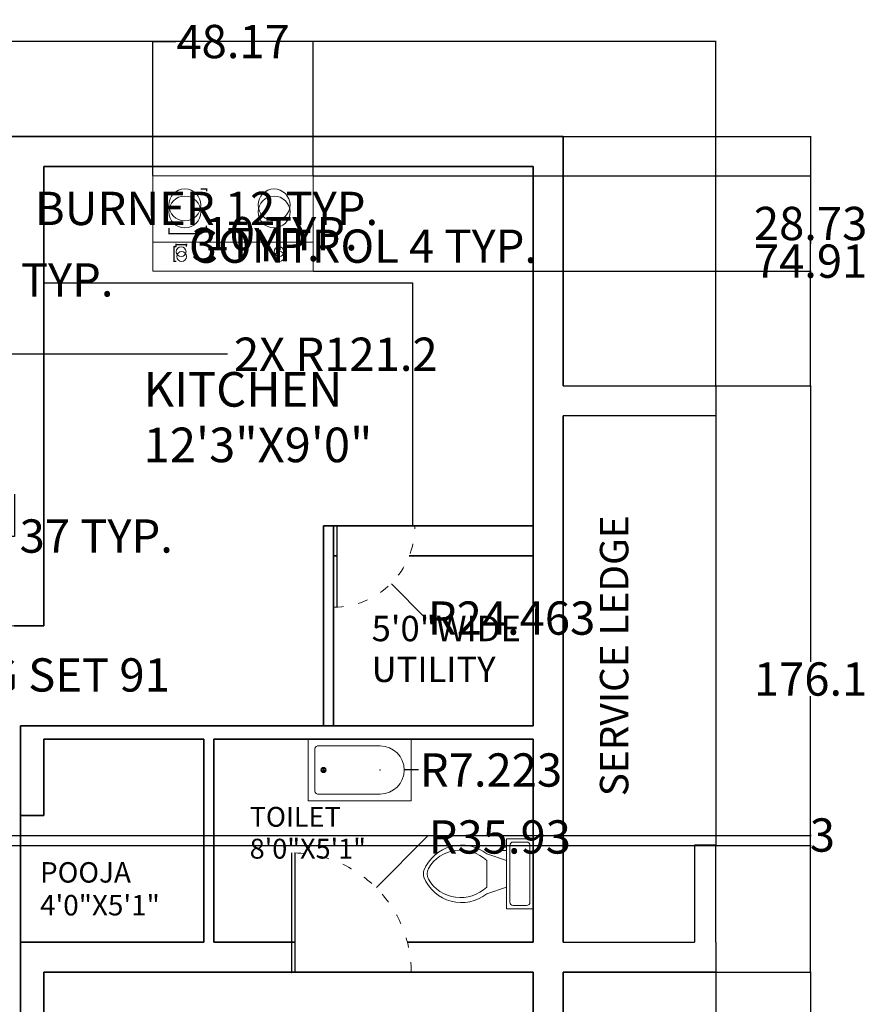
# Model space of a CAD drawing. Units: inches. Extents: x 37 to 687, y -399 to 163.
# Tile 4 of 4: x 432 to 687, y -132 to 163. Entities that reach past the tile are written whole.
import ezdxf

# ---------------------------------------------------------------- set-up
doc = ezdxf.new("R2010")
doc.units = ezdxf.units.IN
doc.header["$MEASUREMENT"] = 0
doc.linetypes.add('ACAD_ISO03W100', pattern=[30, 12, -18])
for name, color, linetype, lineweight in [('A-ANNO-DIMS', 2, 'Continuous', 18), ('A-AREA-IDEN', 7, 'Continuous', 18), ('A-DOOR', 4, 'Continuous', 25), ('A-DOOR-SWNG', 4, 'ACAD_ISO03W100', 13), ('A-EQPM', 8, 'Continuous', 18), ('A-FLOR-CASE', 9, 'Continuous', 25), ('A-FLOR-FIXT', 9, 'Continuous', 18), ('A-FLOR-OTLN', 7, 'Continuous', 25), ('A-WALL', 7, 'Continuous', 35), ('A-WALL-OVHD', 7, 'ACAD_ISO03W100', 18)]:
    doc.layers.add(name, color=color, linetype=linetype, lineweight=lineweight)
doc.styles.get("Standard").update_dxf_attribs({"font": 'arial.ttf'})
doc.dimstyles.get("Standard").update_dxf_attribs({"dimtxt": 10, "dimasz": 0.18, "dimexe": 0.18, "dimexo": 0.0625, "dimgap": 0.09, "dimtad": 0, "dimtih": 1, "dimtoh": 1, "dimdec": 0, "dimzin": 0, "dimdsep": 46, "dimlunit": 3, "dimtxsty": 'Standard', "dimcen": 0.09, "dimadec": 0, "dimazin": 0, "dimtfac": 1, "dimtdec": 0, "dimtofl": 0, "dimtmove": 0, "dimatfit": 3, "dimfxl": 1, "dimtolj": 1, "dimtzin": 0, "dimarcsym": 0})

# ---------------------------------------------------------------- blocks, each defined once
blk = doc.blocks.new('Toilet - top')
for p, q in [((9.5, -6), (9.5, -2)), ((-10, -8.5), (-8, -8.5)), ((-10, -9.5), (-10, -8.5)), ((-8, -8.5), (-8, -8)), ((-7, -8), (-7, -9.5)), ((-4, -8), (-6, -14)), ((4, -8), (6, -14)), ((-7, -9.5), (-10, -9.5)), ((4, -14), (-4, -14))]:
    blk.add_line(p, q)
blk.add_lwpolyline([(10.5, -8), (10.5, 0), (-10.5, 0), (-10.5, -8)], close=True)
for points in [[(-9.5, -2), (-9.5, -6)], [(8.5, -1), (-8.5, -1)], [(-8.5, -7), (8.5, -7)]]:
    blk.add_lwpolyline(points)
for centre, radius, start, end in [((-8.62, -1.88), 0.884, 81.8699, 188.1301), ((8.62, -1.88), 0.884, 351.8699, 98.1301), ((-8.62, -6.12), 0.884, 171.8699, 278.1301), ((8.62, -6.12), 0.884, 261.8699, 8.1301), ((3.52, -21.58), 12.17, 141.4691, 247.9714), ((4.2, -21.82), 11.33, 136.3677, 238.9468), ((-3.52, -21.58), 12.17, 292.0284, 38.5307), ((-4.2, -21.82), 11.33, 301.053, 43.6321), ((0, -27.88), 4, 245.7318, 294.2682), ((0, -29), 4, 254.8605, 285.1395)]:
    blk.add_arc(centre, radius, start, end)
blk = doc.blocks.new('Bath Tub - 26 x 60 in.')
for p, q in [((9, -17), (9, -19)), ((8, -18), (10, -18))]:
    blk.add_line(p, q)
blk.add_lwpolyline([(0, -36), (0, 0), (60, 0), (60, -36)], close=True)
for points in [[(6, -4), (42, -4)], [(4, -30), (4, -6)], [(42, -32), (6, -32)]]:
    blk.add_lwpolyline(points)
for radius in [1.5, 1]:
    blk.add_circle((9, -18), radius)
for centre, radius, start, end in [((5.75, -5.75), 1.77, 81.8699, 188.1301), ((42, -18), 14, 270, 90), ((5.75, -30.25), 1.77, 171.8699, 278.1301)]:
    blk.add_arc(centre, radius, start, end)
blk = doc.blocks.new('COOKTOP-BURNER')
at = {"ltscale": 0.25}
for centre in [(4.78, 6.88), (4.78, 4.77)]:
    blk.add_circle(centre, 4.78, dxfattribs=at)
blk = doc.blocks.new('COOKTOP-CONTROL')
at = {"ltscale": 0.25}
for centre in [(1.47, 2.92), (1.65, 1.47)]:
    blk.add_circle(centre, 1.47, dxfattribs=at)
blk = doc.blocks.new('*D11')
at = {"layer": 'A-ANNO-DIMS', "color": 0, "lineweight": -2, "ltscale": 0.25, "transparency": 16777216}
for p, q in [((347, 88.33), (347, 85.06)), ((368, 88.33), (368, 85.06)), ((347.18, 85.24), (367.82, 85.24)), ((368, 85.24), (368.18, 85.24))]:
    blk.add_line(p, q, dxfattribs=at)
at = {"layer": 'A-ANNO-DIMS', "color": 0, "ltscale": 0.25, "transparency": 16777216}
for points in [[(347.18, 85.27), (347.18, 85.21), (347, 85.24)], [(367.82, 85.27), (367.82, 85.21), (368, 85.24)]]:
    blk.add_solid(points, dxfattribs=at)
at = {"layer": 'Defpoints', "color": 0, "ltscale": 0.25, "transparency": 16777216}
for p in [(347, 88.39), (368, 88.39), (368, 85.24)]:
    blk.add_point(p, dxfattribs=at)
at = {"layer": 'A-ANNO-DIMS', "color": 0, "ltscale": 0.25, "transparency": 16777216, "insert": (416.22, 85.24), "char_height": 10, "attachment_point": 5}
blk.add_mtext('\\A1;CHAIR 21 TYP.', dxfattribs=at)
blk = doc.blocks.new('*D20')
at = {"layer": 'A-ANNO-DIMS', "color": 0, "lineweight": -2, "ltscale": 0.25, "transparency": 16777216}
for p, q in [((394.12, 20.84), (394.12, 8.12)), ((430.79, 20.84), (430.79, 8.12)), ((394.3, 8.3), (430.61, 8.3)), ((430.79, 8.3), (430.97, 8.3))]:
    blk.add_line(p, q, dxfattribs=at)
at = {"layer": 'A-ANNO-DIMS', "color": 0, "ltscale": 0.25, "transparency": 16777216}
for points in [[(394.3, 8.33), (394.3, 8.27), (394.12, 8.3)], [(430.61, 8.33), (430.61, 8.27), (430.79, 8.3)]]:
    blk.add_solid(points, dxfattribs=at)
at = {"layer": 'Defpoints', "color": 0, "ltscale": 0.25, "transparency": 16777216}
for p in [(394.12, 20.9), (430.79, 20.9), (430.79, 8.3)]:
    blk.add_point(p, dxfattribs=at)
at = {"layer": 'A-ANNO-DIMS', "color": 0, "ltscale": 0.25, "transparency": 16777216, "insert": (455.39, 8.3), "char_height": 10, "attachment_point": 5}
blk.add_mtext('\\A1;37 TYP.', dxfattribs=at)
blk = doc.blocks.new('*D21')
at = {"layer": 'A-ANNO-DIMS', "color": 0, "lineweight": -2, "ltscale": 0.25, "transparency": 16777216}
for p, q in [((292.31, -47.01), (292.31, -33.24)), ((292.49, -33.42), (383.13, -33.42)), ((383.31, -47.01), (383.31, -33.24)), ((383.31, -33.42), (383.49, -33.42))]:
    blk.add_line(p, q, dxfattribs=at)
at = {"layer": 'A-ANNO-DIMS', "color": 0, "ltscale": 0.25, "transparency": 16777216}
for points in [[(292.49, -33.39), (292.49, -33.45), (292.31, -33.42)], [(383.13, -33.39), (383.13, -33.45), (383.31, -33.42)]]:
    blk.add_solid(points, dxfattribs=at)
at = {"layer": 'Defpoints', "color": 0, "ltscale": 0.25, "transparency": 16777216}
for p in [(383.31, -33.42), (292.31, -47.07), (383.31, -47.07)]:
    blk.add_point(p, dxfattribs=at)
at = {"layer": 'A-ANNO-DIMS', "color": 0, "ltscale": 0.25, "transparency": 16777216, "insert": (431.44, -33.42), "char_height": 10, "attachment_point": 5}
blk.add_mtext('\\A1;DINING SET 91', dxfattribs=at)
blk = doc.blocks.new('*D23')
at = {"layer": 'A-ANNO-DIMS', "color": 0, "lineweight": -2, "ltscale": 0.25, "transparency": 16777216}
for p, q in [((486.84, 112.53), (488.7, 112.53)), ((488.52, 112.35), (488.52, 111.9)), ((486.84, 100.87), (488.7, 100.87)), ((488.52, 101.05), (488.52, 101.51))]:
    blk.add_line(p, q, dxfattribs=at)
at = {"layer": 'A-ANNO-DIMS', "color": 0, "ltscale": 0.25, "transparency": 16777216}
for points in [[(488.49, 112.35), (488.55, 112.35), (488.52, 112.53)], [(488.49, 101.05), (488.55, 101.05), (488.52, 100.87)]]:
    blk.add_solid(points, dxfattribs=at)
at = {"layer": 'Defpoints', "color": 0, "ltscale": 0.25, "transparency": 16777216}
for p in [(486.77, 112.53), (488.52, 112.53), (486.77, 100.87)]:
    blk.add_point(p, dxfattribs=at)
at = {"layer": 'A-ANNO-DIMS', "color": 0, "ltscale": 0.25, "transparency": 16777216, "insert": (488.52, 106.7), "char_height": 10, "attachment_point": 5}
blk.add_mtext('\\A1;BURNER 12 TYP.', dxfattribs=at)
blk = doc.blocks.new('*D24')
at = {"layer": 'A-ANNO-DIMS', "color": 0, "lineweight": -2, "ltscale": 0.25, "transparency": 16777216}
for p, q in [((477.22, 100.81), (477.22, 98.94)), ((486.77, 100.81), (486.77, 98.94)), ((477.4, 99.12), (486.59, 99.12)), ((486.77, 99.12), (486.95, 99.12))]:
    blk.add_line(p, q, dxfattribs=at)
at = {"layer": 'A-ANNO-DIMS', "color": 0, "ltscale": 0.25, "transparency": 16777216}
for points in [[(477.4, 99.15), (477.4, 99.09), (477.22, 99.12)], [(486.59, 99.15), (486.59, 99.09), (486.77, 99.12)]]:
    blk.add_solid(points, dxfattribs=at)
at = {"layer": 'Defpoints', "color": 0, "ltscale": 0.25, "transparency": 16777216}
for p in [(477.22, 100.87), (486.77, 100.87), (486.77, 99.12)]:
    blk.add_point(p, dxfattribs=at)
at = {"layer": 'A-ANNO-DIMS', "color": 0, "ltscale": 0.25, "transparency": 16777216, "insert": (510.91, 99.12), "char_height": 10, "attachment_point": 5}
blk.add_mtext('\\A1;10 TYP.', dxfattribs=at)
blk = doc.blocks.new('*D25')
at = {"layer": 'A-ANNO-DIMS', "color": 0, "lineweight": -2, "ltscale": 0.25, "transparency": 16777216}
for p, q in [((479.37, 95.18), (478.59, 95.18)), ((478.77, 95.18), (478.77, 95.36)), ((478.77, 95.36), (478.95, 95.36)), ((478.77, 90.97), (478.77, 95)), ((479.37, 90.79), (478.59, 90.79))]:
    blk.add_line(p, q, dxfattribs=at)
at = {"layer": 'A-ANNO-DIMS', "color": 0, "ltscale": 0.25, "transparency": 16777216}
for points in [[(478.74, 95), (478.8, 95), (478.77, 95.18)], [(478.74, 90.97), (478.8, 90.97), (478.77, 90.79)]]:
    blk.add_solid(points, dxfattribs=at)
at = {"layer": 'Defpoints', "color": 0, "ltscale": 0.25, "transparency": 16777216}
for p in [(478.77, 95.18), (479.43, 95.18), (479.43, 90.79)]:
    blk.add_point(p, dxfattribs=at)
at = {"layer": 'A-ANNO-DIMS', "color": 0, "ltscale": 0.25, "transparency": 16777216, "insert": (535.53, 95.36), "char_height": 10, "attachment_point": 5}
blk.add_mtext('\\A1;CONTROL 4 TYP.', dxfattribs=at)
blk = doc.blocks.new('*D26')
at = {"layer": 'A-ANNO-DIMS', "color": 0, "lineweight": -2, "ltscale": 0.25, "transparency": 16777216}
for p, q in [((479.43, 95.24), (479.43, 96.02)), ((479.61, 95.84), (482.37, 95.84)), ((482.55, 95.24), (482.55, 96.02)), ((482.55, 95.84), (482.73, 95.84))]:
    blk.add_line(p, q, dxfattribs=at)
at = {"layer": 'A-ANNO-DIMS', "color": 0, "ltscale": 0.25, "transparency": 16777216}
for points in [[(479.61, 95.87), (479.61, 95.81), (479.43, 95.84)], [(482.37, 95.87), (482.37, 95.81), (482.55, 95.84)]]:
    blk.add_solid(points, dxfattribs=at)
at = {"layer": 'Defpoints', "color": 0, "ltscale": 0.25, "transparency": 16777216}
for p in [(479.43, 95.18), (482.55, 95.84), (482.55, 95.18)]:
    blk.add_point(p, dxfattribs=at)
at = {"layer": 'A-ANNO-DIMS', "color": 0, "ltscale": 0.25, "transparency": 16777216, "insert": (503.27, 95.84), "char_height": 10, "attachment_point": 5}
blk.add_mtext('\\A1;3 TYP.', dxfattribs=at)
blk = doc.blocks.new('*D27')
at = {"layer": 'A-ANNO-DIMS', "color": 0, "lineweight": -2, "ltscale": 0.25, "transparency": 16777216}
for p, q in [((82.29, -12.62), (82.29, 157)), ((82.47, 156.82), (344.98, 156.82)), ((641.3, 156.82), (378.8, 156.82)), ((641.48, 53.47), (641.48, 157))]:
    blk.add_line(p, q, dxfattribs=at)
at = {"layer": 'A-ANNO-DIMS', "color": 0, "ltscale": 0.25, "transparency": 16777216}
for points in [[(82.47, 156.85), (82.47, 156.79), (82.29, 156.82)], [(641.3, 156.85), (641.3, 156.79), (641.48, 156.82)]]:
    blk.add_solid(points, dxfattribs=at)
at = {"layer": 'Defpoints', "color": 0, "ltscale": 0.25, "transparency": 16777216}
for p in [(641.48, 156.82), (641.48, 53.4), (82.29, -12.68)]:
    blk.add_point(p, dxfattribs=at)
at = {"layer": 'A-ANNO-DIMS', "color": 0, "ltscale": 0.25, "transparency": 16777216, "insert": (361.89, 156.82), "char_height": 10, "attachment_point": 5}
blk.add_mtext('\\A1;559.2', dxfattribs=at)
blk = doc.blocks.new('*D33')
at = {"layer": 'A-ANNO-DIMS', "color": 0, "lineweight": -2, "ltscale": 0.25, "transparency": 16777216}
for p, q in [((641.5, -122.75), (641.5, -392.85)), ((595.69, -287.75), (595.69, -392.85)), ((595.87, -392.67), (602.39, -392.67)), ((641.32, -392.67), (634.79, -392.67))]:
    blk.add_line(p, q, dxfattribs=at)
at = {"layer": 'A-ANNO-DIMS', "color": 0, "ltscale": 0.25, "transparency": 16777216}
for points in [[(595.87, -392.64), (595.87, -392.7), (595.69, -392.67)], [(641.32, -392.64), (641.32, -392.7), (641.5, -392.67)]]:
    blk.add_solid(points, dxfattribs=at)
at = {"layer": 'Defpoints', "color": 0, "ltscale": 0.25, "transparency": 16777216}
for p in [(641.5, -122.68), (595.69, -287.68), (641.5, -392.67)]:
    blk.add_point(p, dxfattribs=at)
at = {"layer": 'A-ANNO-DIMS', "color": 0, "ltscale": 0.25, "transparency": 16777216, "insert": (618.59, -392.67), "char_height": 10, "attachment_point": 5}
blk.add_mtext('\\A1;45.81', dxfattribs=at)
blk = doc.blocks.new('*D34')
at = {"layer": 'A-ANNO-DIMS', "color": 0, "lineweight": -2, "ltscale": 0.25, "transparency": 16777216}
for p, q in [((595.75, 128.32), (670.18, 128.32)), ((670, 128.14), (670, 96.06)), ((670, 53.58), (670, 85.66)), ((595.75, 53.4), (670.18, 53.4))]:
    blk.add_line(p, q, dxfattribs=at)
at = {"layer": 'A-ANNO-DIMS', "color": 0, "ltscale": 0.25, "transparency": 16777216}
for points in [[(669.97, 128.14), (670.03, 128.14), (670, 128.32)], [(669.97, 53.58), (670.03, 53.58), (670, 53.4)]]:
    blk.add_solid(points, dxfattribs=at)
at = {"layer": 'Defpoints', "color": 0, "ltscale": 0.25, "transparency": 16777216}
for p in [(595.69, 128.32), (670, 128.32), (595.69, 53.4)]:
    blk.add_point(p, dxfattribs=at)
at = {"layer": 'A-ANNO-DIMS', "color": 0, "ltscale": 0.25, "transparency": 16777216, "insert": (670, 90.86), "char_height": 10, "attachment_point": 5}
blk.add_mtext('\\A1;74.91', dxfattribs=at)
blk = doc.blocks.new('*D35')
at = {"layer": 'A-ANNO-DIMS', "color": 0, "lineweight": -2, "ltscale": 0.25, "transparency": 16777216}
for p, q in [((641.55, 53.4), (670.18, 53.4)), ((670, 53.22), (670, -29.44)), ((670, -122.5), (670, -39.84)), ((641.56, -122.68), (670.18, -122.68))]:
    blk.add_line(p, q, dxfattribs=at)
at = {"layer": 'A-ANNO-DIMS', "color": 0, "ltscale": 0.25, "transparency": 16777216}
for points in [[(669.97, 53.22), (670.03, 53.22), (670, 53.4)], [(669.97, -122.5), (670.03, -122.5), (670, -122.68)]]:
    blk.add_solid(points, dxfattribs=at)
at = {"layer": 'Defpoints', "color": 0, "ltscale": 0.25, "transparency": 16777216}
for p in [(641.48, 53.4), (670, 53.4), (641.5, -122.68)]:
    blk.add_point(p, dxfattribs=at)
at = {"layer": 'A-ANNO-DIMS', "color": 0, "ltscale": 0.25, "transparency": 16777216, "insert": (670, -34.64), "char_height": 10, "attachment_point": 5}
blk.add_mtext('\\A1;176.1', dxfattribs=at)
blk = doc.blocks.new('*D36')
at = {"layer": 'A-ANNO-DIMS', "color": 0, "lineweight": -2, "ltscale": 0.25, "transparency": 16777216}
for p, q in [((595.75, -122.68), (670.18, -122.68)), ((670, -122.86), (670, -199.99)), ((670, -287.5), (670, -210.38)), ((595.75, -287.68), (670.18, -287.68))]:
    blk.add_line(p, q, dxfattribs=at)
at = {"layer": 'A-ANNO-DIMS', "color": 0, "ltscale": 0.25, "transparency": 16777216}
for points in [[(669.97, -122.86), (670.03, -122.86), (670, -122.68)], [(669.97, -287.5), (670.03, -287.5), (670, -287.68)]]:
    blk.add_solid(points, dxfattribs=at)
at = {"layer": 'Defpoints', "color": 0, "ltscale": 0.25, "transparency": 16777216}
for p in [(595.69, -122.68), (670, -122.68), (595.69, -287.68)]:
    blk.add_point(p, dxfattribs=at)
at = {"layer": 'A-ANNO-DIMS', "color": 0, "ltscale": 0.25, "transparency": 16777216, "insert": (670, -205.18), "char_height": 10, "attachment_point": 5}
blk.add_mtext('\\A1;165', dxfattribs=at)
blk = doc.blocks.new('*D38')
at = {"layer": 'A-ANNO-DIMS', "color": 0, "lineweight": -2, "ltscale": 0.25, "transparency": 16777216}
for p, q in [((472.42, 116.59), (472.42, 157)), ((472.6, 156.82), (479.35, 156.82)), ((520.42, 156.82), (513.67, 156.82)), ((520.6, 116.59), (520.6, 157))]:
    blk.add_line(p, q, dxfattribs=at)
at = {"layer": 'A-ANNO-DIMS', "color": 0, "ltscale": 0.25, "transparency": 16777216}
for points in [[(472.6, 156.85), (472.6, 156.79), (472.42, 156.82)], [(520.42, 156.85), (520.42, 156.79), (520.6, 156.82)]]:
    blk.add_solid(points, dxfattribs=at)
at = {"layer": 'Defpoints', "color": 0, "ltscale": 0.25, "transparency": 16777216}
for p in [(520.6, 156.82), (472.42, 116.53), (520.6, 116.53)]:
    blk.add_point(p, dxfattribs=at)
at = {"layer": 'A-ANNO-DIMS', "color": 0, "ltscale": 0.25, "transparency": 16777216, "insert": (496.51, 156.82), "char_height": 10, "attachment_point": 5}
blk.add_mtext('\\A1;48.17', dxfattribs=at)
blk = doc.blocks.new('*D39')
at = {"layer": 'A-ANNO-DIMS', "color": 0, "lineweight": -2, "ltscale": 0.25, "transparency": 16777216}
for p, q in [((520.66, 116.53), (670.18, 116.53)), ((670, 116.35), (670, 107.36)), ((670, 87.98), (670, 96.97)), ((520.66, 87.8), (670.18, 87.8))]:
    blk.add_line(p, q, dxfattribs=at)
at = {"layer": 'A-ANNO-DIMS', "color": 0, "ltscale": 0.25, "transparency": 16777216}
for points in [[(669.97, 116.35), (670.03, 116.35), (670, 116.53)], [(669.97, 87.98), (670.03, 87.98), (670, 87.8)]]:
    blk.add_solid(points, dxfattribs=at)
at = {"layer": 'Defpoints', "color": 0, "ltscale": 0.25, "transparency": 16777216}
for p in [(520.6, 116.53), (520.6, 87.8), (670, 87.8)]:
    blk.add_point(p, dxfattribs=at)
at = {"layer": 'A-ANNO-DIMS', "color": 0, "ltscale": 0.25, "transparency": 16777216, "insert": (670, 102.17), "char_height": 10, "attachment_point": 5}
blk.add_mtext('\\A1;28.73', dxfattribs=at)
blk = doc.blocks.new('*D44')
at = {"layer": 'A-ANNO-DIMS', "color": 0, "lineweight": -2, "ltscale": 0.25, "transparency": 16777216}
for p, q in [((242.75, -81.68), (670.18, -81.68)), ((670, -81.68), (670, -81.5)), ((670, -81.5), (670.18, -81.5)), ((670, -84.5), (670, -81.86)), ((242.75, -84.68), (670.18, -84.68))]:
    blk.add_line(p, q, dxfattribs=at)
at = {"layer": 'A-ANNO-DIMS', "color": 0, "ltscale": 0.25, "transparency": 16777216}
for points in [[(669.97, -81.86), (670.03, -81.86), (670, -81.68)], [(669.97, -84.5), (670.03, -84.5), (670, -84.68)]]:
    blk.add_solid(points, dxfattribs=at)
at = {"layer": 'Defpoints', "color": 0, "ltscale": 0.25, "transparency": 16777216}
for p in [(242.69, -81.68), (670, -81.68), (242.69, -84.68)]:
    blk.add_point(p, dxfattribs=at)
at = {"layer": 'A-ANNO-DIMS', "color": 0, "ltscale": 0.25, "transparency": 16777216, "insert": (673.54, -81.5), "char_height": 10, "attachment_point": 5}
blk.add_mtext('\\A1;3', dxfattribs=at)
blk = doc.blocks.new('*D49')
at = {"layer": 'A-ANNO-DIMS', "color": 0, "lineweight": -2, "ltscale": 0.25, "transparency": 16777216}
for p, q in [((554.69, -82.08), (539.6, -97.22)), ((554.87, -82.08), (554.69, -82.08)), ((514.01, -122.8), (514.19, -122.8)), ((514.1, -122.89), (514.1, -122.71))]:
    blk.add_line(p, q, dxfattribs=at)
at = {"layer": 'A-ANNO-DIMS', "color": 0, "ltscale": 0.25, "transparency": 16777216}
blk.add_solid([(539.57, -97.2), (539.62, -97.25), (539.47, -97.35)], dxfattribs=at)
at = {"layer": 'Defpoints', "color": 0, "ltscale": 0.25, "transparency": 16777216}
for p in [(539.47, -97.35), (514.1, -122.8)]:
    blk.add_point(p, dxfattribs=at)
at = {"layer": 'A-ANNO-DIMS', "color": 0, "ltscale": 0.25, "transparency": 16777216, "insert": (576.62, -82.08), "char_height": 10, "attachment_point": 5}
blk.add_mtext('\\A1;R35.93', dxfattribs=at)
blk = doc.blocks.new('*D53')
at = {"layer": 'A-ANNO-DIMS', "color": 0, "lineweight": -2, "ltscale": 0.25, "transparency": 16777216}
for p, q in [((526.6, 11.36), (526.78, 11.36)), ((526.69, 11.27), (526.69, 11.45)), ((554.33, -16.34), (544.09, -6.08)), ((554.51, -16.34), (554.33, -16.34))]:
    blk.add_line(p, q, dxfattribs=at)
at = {"layer": 'A-ANNO-DIMS', "color": 0, "ltscale": 0.25, "transparency": 16777216}
blk.add_solid([(544.11, -6.06), (544.07, -6.1), (543.97, -5.95)], dxfattribs=at)
at = {"layer": 'Defpoints', "color": 0, "ltscale": 0.25, "transparency": 16777216}
for p in [(526.69, 11.36), (543.97, -5.95)]:
    blk.add_point(p, dxfattribs=at)
at = {"layer": 'A-ANNO-DIMS', "color": 0, "ltscale": 0.25, "transparency": 16777216, "insert": (580.15, -16.34), "char_height": 10, "attachment_point": 5}
blk.add_mtext('\\A1;R24.463', dxfattribs=at)
blk = doc.blocks.new('*D54')
at = {"layer": 'A-ANNO-DIMS', "color": 0, "lineweight": -2, "ltscale": 0.25, "transparency": 16777216}
for p, q in [((300.83, 62.9), (301.01, 62.9)), ((300.92, 62.81), (300.92, 62.99)), ((494.84, 62.9), (422.3, 62.9))]:
    blk.add_line(p, q, dxfattribs=at)
at = {"layer": 'A-ANNO-DIMS', "color": 0, "ltscale": 0.25, "transparency": 16777216}
blk.add_solid([(422.3, 62.93), (422.3, 62.87), (422.12, 62.9)], dxfattribs=at)
at = {"layer": 'Defpoints', "color": 0, "ltscale": 0.25, "transparency": 16777216}
for p in [(300.92, 62.9), (422.12, 62.9)]:
    blk.add_point(p, dxfattribs=at)
at = {"layer": 'A-ANNO-DIMS', "color": 0, "ltscale": 0.25, "transparency": 16777216, "insert": (527.36, 62.9), "char_height": 10, "attachment_point": 5}
blk.add_mtext('\\A1;2X R121.2', dxfattribs=at)
blk = doc.blocks.new('*D61')
at = {"layer": 'A-ANNO-DIMS', "color": 0, "lineweight": -2, "ltscale": 0.25, "transparency": 16777216}
for p, q in [((540.6, -61.97), (540.78, -61.97)), ((540.69, -62.06), (540.69, -61.88)), ((552.24, -61.97), (548.09, -61.97))]:
    blk.add_line(p, q, dxfattribs=at)
at = {"layer": 'A-ANNO-DIMS', "color": 0, "ltscale": 0.25, "transparency": 16777216}
blk.add_solid([(548.09, -61.94), (548.09, -62), (547.91, -61.97)], dxfattribs=at)
at = {"layer": 'Defpoints', "color": 0, "ltscale": 0.25, "transparency": 16777216}
for p in [(540.69, -61.97), (547.91, -61.97)]:
    blk.add_point(p, dxfattribs=at)
at = {"layer": 'A-ANNO-DIMS', "color": 0, "ltscale": 0.25, "transparency": 16777216, "insert": (573.99, -61.97), "char_height": 10, "attachment_point": 5}
blk.add_mtext('\\A1;R7.223', dxfattribs=at)

msp = doc.modelspace()

# ---------------------------------------------------------------- linework, layer by layer
at = {"layer": 'A-DOOR', "ltscale": 0.25}
for p, q in [((526.6852, 11.3154), (526.6852, -13.0996)), ((526.6852, 11.3154), (551.1477, 11.3154)), ((527.6852, 11.3154), (527.6852, -13.0996)), ((514.102, -122.6846), (514.102, -86.8696)), ((515.102, -122.6846), (515.102, -86.8696)), ((514.102, -122.6846), (550.0354, -122.6846))]:
    msp.add_line(p, q, dxfattribs=at)
at = {"layer": 'A-DOOR-SWNG', "ltscale": 0.25}
for centre, radius, start, end in [((526.6852, 11.3629), 24.4626, 270, 359.888685), ((514.102, -122.8031), 35.9336, 0.189046, 90)]:
    msp.add_arc(centre, radius, start, end, dxfattribs=at)
at = {"layer": 'A-EQPM', "ltscale": 0.25}
msp.add_line((472.4229, 96.5649), (520.5957, 96.5649), dxfattribs=at)
msp.add_lwpolyline([(472.4229, 116.5307), (520.5957, 116.5307), (520.5957, 87.801), (472.4229, 87.801)], close=True, dxfattribs=at)
at = {"layer": 'A-FLOR-CASE', "ltscale": 0.25}
for p, q in [((439.6852, 84.3836), (550.3988, 84.3836)), ((550.3988, 84.3836), (550.3988, 11.3154))]:
    msp.add_line(p, q, dxfattribs=at)
at = {"layer": 'A-FLOR-OTLN', "ltscale": 0.25}
for p, q in [((595.6852, 53.4042), (641.4841, 53.4042)), ((641.4841, 53.4042), (641.4841, 44.4042)), ((641.4841, 44.4042), (595.6852, 44.4042)), ((641.4841, 44.4042), (641.4983, -84.5551)), ((641.4983, -84.5551), (635.0829, -84.5551)), ((635.0829, -84.5551), (635.0829, -113.6846)), ((641.4983, -113.6846), (641.4983, -84.5551)), ((595.6852, -113.6846), (635.0829, -113.6846)), ((641.4983, -113.6846), (641.4983, -122.6846)), ((641.4983, -122.6846), (595.6852, -122.6846))]:
    msp.add_line(p, q, dxfattribs=at)
at = {"layer": 'A-WALL'}
for p, q in [((137.6852, 128.3154), (595.6852, 128.3154)), ((439.6852, 128.3154), (586.6852, 128.3154)), ((595.6852, 128.3154), (595.6852, 53.4042)), ((439.6852, 119.3154), (439.6852, -18.6846)), ((439.6852, 119.3154), (586.6852, 119.3154)), ((586.6852, 119.3154), (586.6852, 11.3154)), ((595.6852, 44.4042), (595.6852, -113.6846)), ((586.6852, 11.3154), (523.6852, 11.3154)), ((523.6852, 11.3154), (523.6852, -48.6846)), ((526.6852, 11.3154), (526.6852, -48.6846)), ((586.6852, -48.6846), (586.6852, 11.3154)), ((595.6852, -48.6846), (595.6852, 11.3154)), ((527.6852, 2.3154), (526.6852, 2.3154)), ((586.6852, 2.3154), (549.4131, 2.3154)), ((523.6852, -48.6846), (432.6852, -48.6846)), ((432.6852, -48.6846), (432.6852, -75.6597)), ((490.6852, -48.6846), (526.6852, -48.6846)), ((526.6852, -48.6846), (586.6852, -48.6846)), ((487.6852, -52.6846), (439.6852, -52.6846)), ((439.6852, -52.6846), (439.6852, -75.6597)), ((487.6852, -113.6846), (487.6852, -52.6846)), ((490.6852, -113.6846), (490.6852, -52.6846)), ((490.6852, -52.6846), (526.6852, -52.6846)), ((526.6852, -52.6846), (586.6852, -52.6846)), ((586.6852, -52.6846), (586.6852, -113.6846)), ((595.6852, -52.6846), (595.6852, -113.6846)), ((432.6852, -113.6846), (487.6852, -113.6846)), ((432.6852, -159.3108), (432.6852, -113.6846)), ((515.102, -113.6846), (490.6852, -113.6846)), ((586.6852, -113.6846), (548.8594, -113.6846)), ((439.6852, -122.6846), (487.6852, -122.6846)), ((439.6852, -159.3108), (439.6852, -122.6846)), ((493.7776, -122.6846), (487.6852, -122.6846)), ((586.6852, -122.6846), (490.6852, -122.6846)), ((586.6852, -122.6846), (586.6852, -278.6846)), ((595.6852, -122.6846), (595.6852, -278.6846)), ((595.6852, -122.6846), (595.6852, -287.6846))]:
    msp.add_line(p, q, dxfattribs=at)
at = {"layer": 'A-WALL', "ltscale": 0.25}
for p, q in [((439.6852, -18.6846), (430.6852, -18.6846)), ((439.6852, -75.6597), (432.6852, -75.6597)), ((432.6852, -75.6597), (432.6852, -113.6846))]:
    msp.add_line(p, q, dxfattribs=at)
at = {"layer": 'A-WALL-OVHD', "ltscale": 0.25}
msp.add_line((439.6852, -18.6846), (283.6852, -18.6846), dxfattribs=at)

# ---------------------------------------------------------------- block references
at = {"layer": 'A-EQPM'}
for name, p in [('COOKTOP-BURNER', (477.224, 100.871)), ('COOKTOP-BURNER', (504.0398, 100.871)), ('COOKTOP-CONTROL', (479.43, 90.786))]:
    msp.add_blockref(name, p, dxfattribs=at)
at = {"layer": 'A-EQPM', "rotation": 180}
msp.add_blockref('COOKTOP-CONTROL', (511.9738, 95.1775), dxfattribs=at)
at = {"layer": 'A-FLOR-FIXT', "ltscale": 0.25, "xscale": 0.5159301814603471, "yscale": 0.5159301814603471, "zscale": 0.5159301814603471}
msp.add_blockref('Bath Tub - 26 x 60 in.', (519.0182, -52.6846), dxfattribs=at)
at = {"layer": 'A-FLOR-FIXT', "ltscale": 0.25, "rotation": 270}
msp.add_blockref('Toilet - top', (586.6852, -93.1539), dxfattribs=at)

# ---------------------------------------------------------------- texts
at = {"layer": 'A-AREA-IDEN', "ltscale": 0.25}
for s, height, p in [('KITCHEN', 10.38481, (469.6214, 47.1592)), ('12\'3"X9\'0"', 10.38481, (469.6214, 30.4769)), ('5\'0"WIDE', 7.62722, (538.1191, -23.2951)), ('UTILITY', 7.62722, (538.1191, -35.5475)), ('TOILET', 5.96011, (501.4886, -79.0098)), ('8\'0"X5\'1"', 5.96011, (501.4886, -88.5842)), ('POOJA', 6.13746, (438.5083, -95.789)), ('4\'0"X5\'1"', 6.13746, (438.5083, -105.6483))]:
    msp.add_text(s, height=height, dxfattribs=at).set_placement(p)
msp.add_text('SERVICE LEDGE', height=8.545704, rotation=90, dxfattribs=at).set_placement((615.2502, -69.8635))

# ---------------------------------------------------------------- dimensions: what is measured, and where the dimension line sits
at = {"layer": 'A-ANNO-DIMS', "ltscale": 0.25}
for base, p1, p2, override, picture, middle in [((641.4841, 156.8154), (82.2949, -12.6846), (641.4841, 53.4042), {"dimdec": 1, "dimlfac": 1, "dimrnd": 0, "dimzin": 0, "dimdsep": 46, "dimlunit": 2}, '*D27', (361.8895, 156.8154)), ((520.5957, 156.8154), (472.4229, 116.5307), (520.5957, 116.5307), {"dimdec": 2, "dimlfac": 1, "dimrnd": 0, "dimzin": 0, "dimdsep": 46, "dimlunit": 2}, '*D38', (496.5093, 156.8154)), ((641.4983, -392.6681), (595.6852, -287.6846), (641.4983, -122.6846), {"dimdec": 2, "dimlfac": 1, "dimrnd": 0, "dimzin": 0, "dimdsep": 46, "dimlunit": 2}, '*D33', (618.5917, -392.6681))]:
    dim = msp.add_linear_dim(base=base, p1=p1, p2=p2, dimstyle='Standard', override=override, dxfattribs=at)
    dim.commit()
    dim.dimension.update_dxf_attribs({"geometry": picture, "text_midpoint": middle})
for base, p1, p2, text, picture, middle in [((488.5239, 112.5311), (486.7749, 100.8705), (486.7749, 112.5311), 'BURNER <> TYP.', '*D23', (488.5239, 106.7008)), ((478.7711, 95.1774), (479.4298, 90.7861), (479.4298, 95.1774), 'CONTROL <> TYP.', '*D25', (535.5281, 95.3574))]:
    dim = msp.add_linear_dim(base=base, p1=p1, p2=p2, angle=90, text=text, dimstyle='Standard', override={"dimdec": 0, "dimlfac": 1, "dimrnd": 0, "dimzin": 0, "dimdsep": 46, "dimlunit": 2}, dxfattribs=at)
    dim.commit()
    dim.dimension.update_dxf_attribs({"geometry": picture, "text_midpoint": middle})
for base, p1, p2, override, picture, middle in [((669.9983, 128.3154), (595.6852, 53.4042), (595.6852, 128.3154), {"dimdec": 2, "dimlfac": 1, "dimrnd": 0, "dimzin": 0, "dimdsep": 46, "dimlunit": 2}, '*D34', (669.9983, 90.8598)), ((669.9983, 87.801), (520.5957, 116.5307), (520.5957, 87.801), {"dimdec": 2, "dimlfac": 1, "dimrnd": 0, "dimzin": 0, "dimdsep": 46, "dimlunit": 2}, '*D39', (669.9983, 102.1658)), ((669.9983, 53.4042), (641.4983, -122.6846), (641.4841, 53.4042), {"dimdec": 1, "dimlfac": 1, "dimrnd": 0, "dimzin": 0, "dimdsep": 46, "dimlunit": 2}, '*D35', (669.9983, -34.6402)), ((669.9983, -81.6846), (242.6852, -84.6846), (242.6852, -81.6846), {"dimdec": 0, "dimlfac": 1, "dimrnd": 0, "dimzin": 0, "dimdsep": 46, "dimlunit": 2}, '*D44', (673.5425, -81.5046)), ((669.9983, -122.6846), (595.6852, -287.6846), (595.6852, -122.6846), {"dimdec": 0, "dimlfac": 1, "dimrnd": 0, "dimzin": 0, "dimdsep": 46, "dimlunit": 2}, '*D36', (669.9983, -205.1846))]:
    dim = msp.add_linear_dim(base=base, p1=p1, p2=p2, angle=90, dimstyle='Standard', override=override, dxfattribs=at)
    dim.commit()
    dim.dimension.update_dxf_attribs({"geometry": picture, "text_midpoint": middle})
for base, p1, p2, text, picture, middle in [((486.7749, 99.1214), (477.224, 100.8705), (486.7749, 100.8705), '<> TYP.', '*D24', (510.9125, 99.1214)), ((482.5487, 95.8362), (479.4298, 95.1774), (482.5487, 95.1774), '<> TYP.', '*D26', (503.2689, 95.8362)), ((368.0001, 85.2436), (347.0001, 88.3936), (368.0001, 88.3936), 'CHAIR <> TYP.', '*D11', (416.2237, 85.2436)), ((430.7856, 8.2991), (394.1189, 20.8991), (430.7856, 20.8991), '<> TYP.', '*D20', (455.3905, 8.2991)), ((383.3108, -33.4222), (292.3108, -47.0722), (383.3108, -47.0722), 'DINING SET <>', '*D21', (431.4423, -33.4222))]:
    dim = msp.add_linear_dim(base=base, p1=p1, p2=p2, text=text, dimstyle='Standard', override={"dimdec": 0, "dimlfac": 1, "dimrnd": 0, "dimzin": 0, "dimdsep": 46, "dimlunit": 2}, dxfattribs=at)
    dim.commit()
    dim.dimension.update_dxf_attribs({"geometry": picture, "text_midpoint": middle})
dim = msp.add_radius_dim(center=(300.9221, 62.8991), mpoint=(422.1189, 62.899), text='2X <>', dimstyle='Standard', override={"dimdec": 1, "dimlfac": 1, "dimrnd": 0, "dimzin": 0, "dimdsep": 46, "dimlunit": 2}, dxfattribs=at)
dim.commit()
dim.dimension.update_dxf_attribs({"geometry": '*D54', "text_midpoint": (494.837, 62.8989), "dimtype": 164})
for center, mpoint, override, picture, middle in [((526.6852, 11.3629), (543.9658, -5.9518), {"dimdec": 3, "dimlfac": 1, "dimrnd": 0, "dimzin": 0, "dimdsep": 46, "dimlunit": 2}, '*D53', (580.1464, -16.3406)), ((540.6873, -61.9713), (547.9103, -61.971), {"dimdec": 3, "dimlfac": 1, "dimrnd": 0, "dimzin": 0, "dimdsep": 46, "dimlunit": 2}, '*D61', (552.2441, -61.9708)), ((514.102, -122.8031), (539.4688, -97.3522), {"dimdec": 2, "dimlfac": 1, "dimrnd": 0, "dimzin": 0, "dimdsep": 46, "dimlunit": 2}, '*D49', (576.6164, -82.0817))]:
    dim = msp.add_radius_dim(center=center, mpoint=mpoint, dimstyle='Standard', override=override, dxfattribs=at)
    dim.commit()
    dim.dimension.update_dxf_attribs({"geometry": picture, "text_midpoint": middle, "dimtype": 164})

doc.saveas('drawing.dxf')
